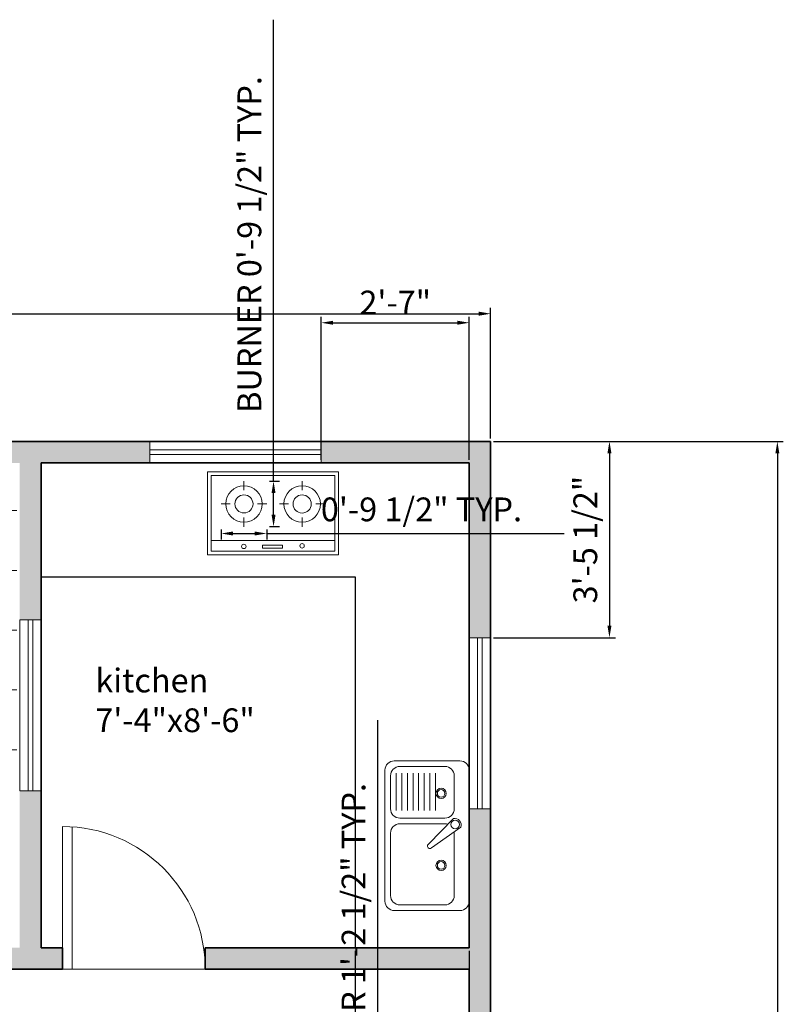
# Model space of a CAD drawing. Units: inches. Extents: x 2576 to 2974, y 2059 to 2656.
# Tile 4 of 4: x 2814 to 2974, y 2448 to 2656. Entities that reach past the tile are written whole.
import ezdxf

# ---------------------------------------------------------------- set-up
doc = ezdxf.new("R2010")
doc.units = ezdxf.units.IN
for name, color, linetype, lineweight in [('A-ANNO-DIMS', 101, 'Continuous', 18), ('A-AREA-IDEN', 101, 'Continuous', 18), ('A-EQPM', 195, 'Continuous', 18), ('A-FLOR-CASE', 143, 'Continuous', 25), ('A-FLOR-FIXT', 195, 'Continuous', 18), ('A-FLOR-PATT', 195, 'Continuous', 13), ('A-WALL-PATT', 233, 'Continuous', 13), ('doors', 235, 'Continuous', 18), ('wall', 143, 'Continuous', 35), ('windows', 85, 'Continuous', 18)]:
    doc.layers.add(name, color=color, linetype=linetype, lineweight=lineweight)
doc.styles.get("Standard").update_dxf_attribs({"font": 'txt', "height": 5})
doc.dimstyles.new('ISO-25', dxfattribs={"dimtxt": 5, "dimasz": 2.5, "dimexe": 1.25, "dimexo": 0.625, "dimtad": 1, "dimlunit": 3, "dimtxsty": 'Standard', "dimcen": 2.5, "dimadec": 0, "dimazin": 0, "dimtfac": 1, "dimtmove": 0, "dimatfit": 3, "dimfxl": 1, "dimarcsym": 0})

# ---------------------------------------------------------------- blocks, each defined once
blk = doc.blocks.new('*D2')
at = {"layer": 'A-ANNO-DIMS', "color": 0, "lineweight": -2, "transparency": 16777216}
for p, q in [((2612.56, 2567.5), (2612.56, 2595)), ((2615.06, 2593.75), (2910.06, 2593.75)), ((2912.56, 2567.5), (2912.56, 2595))]:
    blk.add_line(p, q, dxfattribs=at)
at = {"layer": 'A-ANNO-DIMS', "color": 0, "transparency": 16777216}
for points in [[(2615.06, 2594.17), (2615.06, 2593.33), (2612.56, 2593.75)], [(2910.06, 2594.17), (2910.06, 2593.33), (2912.56, 2593.75)]]:
    blk.add_solid(points, dxfattribs=at)
at = {"layer": 'Defpoints', "color": 0, "transparency": 16777216}
for p in [(2912.56, 2593.75), (2612.56, 2566.88), (2912.56, 2566.88)]:
    blk.add_point(p, dxfattribs=at)
at = {"layer": 'A-ANNO-DIMS', "color": 0, "transparency": 16777216, "insert": (2762.56, 2597.35), "char_height": 5, "attachment_point": 5}
blk.add_mtext("25'", dxfattribs=at)
blk = doc.blocks.new('*D3')
at = {"layer": 'A-ANNO-DIMS', "color": 0, "lineweight": -2, "transparency": 16777216}
for p, q in [((2913.18, 2566.88), (2974.08, 2566.88)), ((2972.83, 2564.38), (2972.83, 2089.38)), ((2913.18, 2086.88), (2974.08, 2086.88))]:
    blk.add_line(p, q, dxfattribs=at)
at = {"layer": 'A-ANNO-DIMS', "color": 0, "transparency": 16777216}
for points in [[(2972.41, 2564.38), (2973.24, 2564.38), (2972.83, 2566.88)], [(2972.41, 2089.38), (2973.24, 2089.38), (2972.83, 2086.88)]]:
    blk.add_solid(points, dxfattribs=at)
at = {"layer": 'Defpoints', "color": 0, "transparency": 16777216}
for p in [(2912.56, 2566.88), (2912.56, 2086.88), (2972.83, 2086.88)]:
    blk.add_point(p, dxfattribs=at)
at = {"layer": 'A-ANNO-DIMS', "color": 0, "transparency": 16777216, "insert": (2969.23, 2326.88), "char_height": 5, "attachment_point": 5, "rotation": 90}
blk.add_mtext("40'", dxfattribs=at)
blk = doc.blocks.new('DOOR-SWING-30IN')
for p, q in [((0, 30), (30, 30)), ((30, 30), (30, 0)), ((0.07, 28), (30, 28))]:
    blk.add_line(p, q)
blk.add_arc((30, 30), 30, 180, 270)
blk = doc.blocks.new('WINDOW-36IN')
for p, q in [((0, 36), (0, 0)), ((4.5, 36), (0, 36)), ((1.75, 36), (1.75, 0)), ((2.75, 36), (2.75, 0)), ((4.5, 0), (4.5, 36)), ((0, 0), (4.5, 0))]:
    blk.add_line(p, q)
blk = doc.blocks.new('COOKTOP-BURNER')
for p, q in [((4.79, 9.57), (4.79, 7.66)), ((0, 4.79), (1.91, 4.79)), ((7.66, 4.79), (9.57, 4.79)), ((4.79, 1.91), (4.79, 0))]:
    blk.add_line(p, q)
for radius in [3.83, 1.91]:
    blk.add_circle((4.79, 4.79), radius)
blk = doc.blocks.new('*D15')
at = {"layer": 'A-ANNO-DIMS', "color": 0, "lineweight": -2, "transparency": 16777216}
for p, q in [((2888.82, 2390.91), (2888.82, 2508.23)), ((2887.27, 2390.91), (2890.07, 2390.91)), ((2888.82, 2378.9), (2888.82, 2388.41)), ((2887.27, 2376.4), (2890.07, 2376.4))]:
    blk.add_line(p, q, dxfattribs=at)
at = {"layer": 'A-ANNO-DIMS', "color": 0, "transparency": 16777216}
for points in [[(2888.4, 2388.41), (2889.23, 2388.41), (2888.82, 2390.91)], [(2888.4, 2378.9), (2889.23, 2378.9), (2888.82, 2376.4)]]:
    blk.add_solid(points, dxfattribs=at)
at = {"layer": 'Defpoints', "color": 0, "transparency": 16777216}
for p in [(2886.64, 2390.91), (2888.82, 2390.91), (2886.64, 2376.4)]:
    blk.add_point(p, dxfattribs=at)
at = {"layer": 'A-ANNO-DIMS', "color": 0, "transparency": 16777216, "insert": (2884.38, 2450.82), "char_height": 5, "attachment_point": 5, "rotation": 90}
blk.add_mtext('DINING CHAIR 1\'-2 1/2" TYP.', dxfattribs=at)
blk = doc.blocks.new('*D17')
at = {"layer": 'A-ANNO-DIMS', "color": 0, "lineweight": -2, "transparency": 16777216}
for p, q in [((2866.92, 2558.52), (2866.92, 2655.6)), ((2866.1, 2558.52), (2868.17, 2558.52)), ((2866.92, 2551.45), (2866.92, 2556.02)), ((2866.1, 2548.95), (2868.17, 2548.95))]:
    blk.add_line(p, q, dxfattribs=at)
at = {"layer": 'A-ANNO-DIMS', "color": 0, "transparency": 16777216}
for points in [[(2866.5, 2556.02), (2867.33, 2556.02), (2866.92, 2558.52)], [(2866.5, 2551.45), (2867.33, 2551.45), (2866.92, 2548.95)]]:
    blk.add_solid(points, dxfattribs=at)
at = {"layer": 'Defpoints', "color": 0, "transparency": 16777216}
for p in [(2865.48, 2558.52), (2866.92, 2558.52), (2865.48, 2548.95)]:
    blk.add_point(p, dxfattribs=at)
at = {"layer": 'A-ANNO-DIMS', "color": 0, "transparency": 16777216, "insert": (2862.48, 2608.31), "char_height": 5, "attachment_point": 5, "rotation": 90}
blk.add_mtext('BURNER 0\'-9 1/2" TYP.', dxfattribs=at)
blk = doc.blocks.new('*D18')
at = {"layer": 'A-ANNO-DIMS', "color": 0, "lineweight": -2, "transparency": 16777216}
for p, q in [((2855.91, 2548.32), (2855.91, 2546.26)), ((2865.48, 2548.32), (2865.48, 2546.26)), ((2858.41, 2547.51), (2862.98, 2547.51)), ((2865.48, 2547.51), (2928.04, 2547.51))]:
    blk.add_line(p, q, dxfattribs=at)
at = {"layer": 'A-ANNO-DIMS', "color": 0, "transparency": 16777216}
for points in [[(2858.41, 2547.93), (2858.41, 2547.09), (2855.91, 2547.51)], [(2862.98, 2547.93), (2862.98, 2547.09), (2865.48, 2547.51)]]:
    blk.add_solid(points, dxfattribs=at)
at = {"layer": 'Defpoints', "color": 0, "transparency": 16777216}
for p in [(2855.91, 2548.95), (2865.48, 2548.95), (2865.48, 2547.51)]:
    blk.add_point(p, dxfattribs=at)
at = {"layer": 'A-ANNO-DIMS', "color": 0, "transparency": 16777216, "insert": (2898.01, 2551.94), "char_height": 5, "attachment_point": 5}
blk.add_mtext('0\'-9 1/2" TYP.', dxfattribs=at)
blk = doc.blocks.new('*D26')
at = {"layer": 'A-ANNO-DIMS', "color": 0, "lineweight": -2, "transparency": 16777216}
for p, q in [((2876.94, 2563), (2876.94, 2593.1)), ((2879.44, 2591.85), (2905.56, 2591.85)), ((2908.06, 2563), (2908.06, 2593.1))]:
    blk.add_line(p, q, dxfattribs=at)
at = {"layer": 'A-ANNO-DIMS', "color": 0, "transparency": 16777216}
for points in [[(2879.44, 2592.27), (2879.44, 2591.43), (2876.94, 2591.85)], [(2905.56, 2592.27), (2905.56, 2591.43), (2908.06, 2591.85)]]:
    blk.add_solid(points, dxfattribs=at)
at = {"layer": 'Defpoints', "color": 0, "transparency": 16777216}
for p in [(2908.06, 2591.85), (2876.94, 2562.38), (2908.06, 2562.38)]:
    blk.add_point(p, dxfattribs=at)
at = {"layer": 'A-ANNO-DIMS', "color": 0, "transparency": 16777216, "insert": (2892.5, 2595.45), "char_height": 5, "attachment_point": 5}
blk.add_mtext('2\'-7"', dxfattribs=at)
blk = doc.blocks.new('*D28')
at = {"layer": 'A-ANNO-DIMS', "color": 0, "lineweight": -2, "transparency": 16777216}
for p, q in [((2913.18, 2566.88), (2938.78, 2566.88)), ((2937.53, 2564.38), (2937.53, 2528.09)), ((2913.18, 2525.59), (2938.78, 2525.59))]:
    blk.add_line(p, q, dxfattribs=at)
at = {"layer": 'A-ANNO-DIMS', "color": 0, "transparency": 16777216}
for points in [[(2937.11, 2564.38), (2937.95, 2564.38), (2937.53, 2566.88)], [(2937.11, 2528.09), (2937.95, 2528.09), (2937.53, 2525.59)]]:
    blk.add_solid(points, dxfattribs=at)
at = {"layer": 'Defpoints', "color": 0, "transparency": 16777216}
for p in [(2912.56, 2566.88), (2912.56, 2525.59), (2937.53, 2525.59)]:
    blk.add_point(p, dxfattribs=at)
at = {"layer": 'A-ANNO-DIMS', "color": 0, "transparency": 16777216, "insert": (2933.1, 2546.23), "char_height": 5, "attachment_point": 5, "rotation": 90}
blk.add_mtext('3\'-5 1/2"', dxfattribs=at)
blk = doc.blocks.new('*D38')
at = {"layer": 'A-ANNO-DIMS', "color": 0, "lineweight": -2, "transparency": 16777216}
for p, q in [((2884.06, 2459.75), (2884.06, 2060.65)), ((2908.06, 2459.75), (2908.06, 2060.65)), ((2886.56, 2061.9), (2905.56, 2061.9))]:
    blk.add_line(p, q, dxfattribs=at)
at = {"layer": 'A-ANNO-DIMS', "color": 0, "transparency": 16777216}
for points in [[(2886.56, 2062.32), (2886.56, 2061.48), (2884.06, 2061.9)], [(2905.56, 2062.32), (2905.56, 2061.48), (2908.06, 2061.9)]]:
    blk.add_solid(points, dxfattribs=at)
at = {"layer": 'Defpoints', "color": 0, "transparency": 16777216}
for p in [(2884.06, 2460.38), (2908.06, 2460.38), (2908.06, 2061.9)]:
    blk.add_point(p, dxfattribs=at)
at = {"layer": 'A-ANNO-DIMS', "color": 0, "transparency": 16777216, "insert": (2896.06, 2065.5), "char_height": 5, "attachment_point": 5}
blk.add_mtext('2\'-0"', dxfattribs=at)

msp = doc.modelspace()

# ---------------------------------------------------------------- hatches: boundary and pattern name
at = {"layer": 'A-FLOR-PATT'}
h = msp.add_hatch(dxfattribs=at)
h.set_pattern_fill('ANGLE', color=256, scale=1.8)
h.set_pattern_definition([(0, (0, 0), (0, 12.573), [9.144, -3.429]), (90, (0, 0), (-12.573, 8e-16), [9.144, -3.429])])
h.paths.add_polyline_path([(2813.556, 2562.376), (2741.556, 2562.376), (2741.556, 2493.376), (2813.556, 2493.376), (2813.556, 2529.376)])
h.paths.add_polyline_path([(2750.035, 2495.142), (2809.21, 2495.142), (2809.21, 2502.647), (2750.035, 2502.647)], flags=24)
h.paths.add_polyline_path([(2741.924, 2553.087), (2815.278, 2553.087), (2815.278, 2560.74), (2741.924, 2560.74)], flags=9)
at = {"layer": 'A-WALL-PATT'}
h = msp.add_hatch(color=256, dxfattribs=at)
h.dxf.hatch_style = 1
h.paths.add_polyline_path([(2726.595, 2349.876), (2706.556, 2349.876), (2706.556, 2381.376), (2702.056, 2381.376), (2702.056, 2349.876), (2617.056, 2349.876), (2617.056, 2370.876), (2612.556, 2370.876), (2612.556, 2287.457), (2617.056, 2287.457), (2617.056, 2345.376), (2726.595, 2345.376)])
h.paths.add_polyline_path([(2823.556, 2345.376), (2828.056, 2345.376), (2828.056, 2349.876), (2808.018, 2349.876), (2808.018, 2345.376), (2819.056, 2345.376), (2819.056, 2206.376), (2748.056, 2206.376), (2748.056, 2201.876), (2819.056, 2201.876), (2819.056, 2159.528), (2823.556, 2159.528)])
h.paths.add_polyline_path([(2634.556, 2206.376), (2617.056, 2206.376), (2617.056, 2239.457), (2612.556, 2239.457), (2612.556, 2086.876), (2696.755, 2086.876), (2696.755, 2091.376), (2617.056, 2091.376), (2617.056, 2201.876), (2634.556, 2201.876)])
h.paths.add_polyline_path([(2688.056, 2206.376), (2670.556, 2206.376), (2670.556, 2201.876), (2688.056, 2201.876)], flags=17)
h.paths.add_polyline_path([(2832.708, 2091.376), (2732.755, 2091.376), (2732.755, 2086.876), (2832.708, 2086.876)])
h.paths.add_polyline_path([(2823.556, 2159.528), (2819.056, 2159.528), (2819.056, 2128.522), (2823.556, 2124.554)])
h.paths.add_polyline_path([(2840.936, 2566.876), (2689.889, 2566.876), (2689.889, 2562.376), (2730.206, 2562.376), (2737.056, 2562.376), (2737.056, 2529.376), (2741.556, 2529.376), (2741.556, 2562.376), (2813.556, 2562.376), (2813.556, 2529.376), (2818.056, 2529.376), (2818.056, 2562.376), (2840.936, 2562.376)])
h.paths.add_polyline_path([(2653.889, 2566.876), (2612.556, 2566.876), (2612.556, 2509.376), (2617.056, 2509.376), (2617.056, 2562.376), (2653.889, 2562.376)])
h.paths.add_polyline_path([(2822.556, 2460.376), (2818.056, 2460.376), (2818.056, 2493.376), (2813.556, 2493.376), (2813.556, 2460.376), (2809.817, 2460.376), (2809.817, 2455.876), (2822.556, 2455.876)])
h.paths.add_polyline_path([(2912.556, 2489.593), (2908.056, 2489.593), (2908.056, 2470.164), (2908.056, 2460.376), (2852.556, 2460.376), (2852.556, 2455.876), (2908.056, 2455.876), (2908.056, 2349.876), (2858.056, 2349.876), (2858.056, 2345.376), (2908.056, 2345.376), (2908.056, 2285.493), (2912.556, 2285.493)])
h.paths.add_polyline_path([(2749.817, 2460.376), (2741.556, 2460.376), (2741.556, 2493.376), (2737.056, 2493.376), (2737.056, 2450.376), (2741.556, 2450.376), (2741.556, 2455.876), (2749.817, 2455.876)])
h.paths.add_polyline_path([(2741.556, 2420.376), (2711.556, 2420.376), (2617.056, 2420.376), (2617.056, 2473.376), (2612.556, 2473.376), (2612.556, 2394.876), (2617.056, 2394.876), (2617.056, 2415.876), (2702.056, 2415.876), (2702.056, 2411.376), (2706.556, 2411.376), (2706.556, 2415.876), (2741.556, 2415.876)])
h.paths.add_polyline_path([(2912.556, 2566.876), (2876.936, 2566.876), (2876.936, 2562.376), (2908.056, 2562.376), (2908.056, 2525.593), (2912.556, 2525.593)])
h.paths.add_polyline_path([(2741.924, 2553.087), (2815.278, 2553.087), (2815.278, 2560.74), (2741.924, 2560.74)], flags=25)

# ---------------------------------------------------------------- linework, layer by layer
at = {"layer": 'A-EQPM'}
for p, q in [((2853.037, 2560.51), (2853.037, 2543.01)), ((2853.037, 2560.51), (2880.593, 2560.51)), ((2880.593, 2560.51), (2880.593, 2543.01)), ((2853.803, 2559.744), (2853.803, 2543.776)), ((2853.803, 2559.744), (2879.828, 2559.744)), ((2879.828, 2559.744), (2879.828, 2543.776)), ((2853.803, 2546.073), (2879.828, 2546.073)), ((2853.803, 2543.776), (2879.828, 2543.776)), ((2864.589, 2545.054), (2868.81, 2545.054)), ((2864.589, 2544.447), (2864.589, 2545.054)), ((2868.81, 2544.447), (2864.589, 2544.447)), ((2868.81, 2545.054), (2868.81, 2544.447)), ((2853.037, 2543.01), (2880.593, 2543.01))]:
    msp.add_line(p, q, dxfattribs=at)
for centre in [(2860.672, 2544.784), (2872.928, 2544.919)]:
    msp.add_circle(centre, 0.459, dxfattribs=at)
at = {"layer": 'A-FLOR-CASE'}
for p, q in [((2818.056, 2538.376), (2884.056, 2538.376)), ((2884.056, 2538.376), (2884.056, 2460.376))]:
    msp.add_line(p, q, dxfattribs=at)
at = {"layer": 'A-FLOR-FIXT'}
for p, q in [((2906.088, 2499.691), (2892.308, 2499.691)), ((2902.938, 2498.51), (2893.489, 2498.51)), ((2890.34, 2497.723), (2890.34, 2470.164)), ((2891.521, 2496.542), (2891.521, 2489.601)), ((2892.695, 2489.215), (2892.695, 2497.104)), ((2893.876, 2489.215), (2893.876, 2497.104)), ((2895.058, 2489.215), (2895.058, 2497.104)), ((2896.239, 2489.215), (2896.239, 2497.104)), ((2897.42, 2489.215), (2897.42, 2497.104)), ((2898.601, 2489.215), (2898.601, 2497.104)), ((2899.782, 2489.215), (2899.782, 2497.104)), ((2900.963, 2489.215), (2900.963, 2497.104)), ((2904.907, 2496.542), (2904.907, 2489.601)), ((2908.056, 2470.164), (2908.056, 2497.723)), ((2902.938, 2487.632), (2893.489, 2487.632)), ((2902.938, 2486.451), (2893.489, 2486.451)), ((2904.755, 2487.545), (2899.466, 2482.167)), ((2906.291, 2485.749), (2900.156, 2481.361)), ((2891.521, 2484.483), (2891.521, 2471.345)), ((2904.907, 2471.345), (2904.907, 2484.483)), ((2893.489, 2469.376), (2902.938, 2469.376)), ((2892.308, 2468.195), (2906.088, 2468.195))]:
    msp.add_line(p, q, dxfattribs=at)
for centre, radius in [((2902.145, 2492.844), 1.081), ((2902.145, 2492.844), 0.788), ((2905.104, 2486.289), 0.892), ((2902.145, 2477.698), 1.081), ((2902.145, 2477.698), 0.788)]:
    msp.add_circle(centre, radius, dxfattribs=at)
for centre, radius, start, end in [((2892.308, 2497.723), 1.968, 90, 180), ((2893.489, 2496.542), 1.968, 90, 180), ((2902.938, 2496.542), 1.968, 0, 90), ((2906.088, 2497.723), 1.968, 0, 90), ((2893.489, 2489.601), 1.968, 180, 270), ((2902.938, 2489.601), 1.968, 270, 0), ((2893.489, 2484.483), 1.968, 90, 180), ((2902.938, 2484.483), 1.968, 71.10956, 90), ((2905.005, 2486.204), 1.364, 340.52706, 100.52706), ((2902.938, 2484.483), 1.968, 0, 7.6978), ((2899.805, 2481.759), 0.531, 129.73777, 311.31634), ((2893.489, 2471.345), 1.968, 180, 270), ((2902.938, 2471.345), 1.968, 270, 0), ((2892.308, 2470.164), 1.968, 180, 270), ((2906.088, 2470.164), 1.968, 270, 0)]:
    msp.add_arc(centre, radius, start, end, dxfattribs=at)
at = {"layer": 'wall'}
for p, q in [((2612.556, 2566.876), (2912.556, 2566.876)), ((2912.556, 2566.876), (2912.556, 2086.876)), ((2818.056, 2460.376), (2818.056, 2562.376)), ((2818.056, 2562.376), (2908.056, 2562.376)), ((2908.056, 2562.376), (2908.056, 2460.376)), ((2818.056, 2460.376), (2822.556, 2460.376)), ((2822.556, 2460.376), (2822.556, 2455.876)), ((2852.556, 2460.376), (2852.556, 2455.876)), ((2852.556, 2460.376), (2908.056, 2460.376)), ((2809.817, 2455.876), (2822.556, 2455.876)), ((2852.556, 2455.876), (2908.056, 2455.876)), ((2908.056, 2455.876), (2908.056, 2349.876))]:
    msp.add_line(p, q, dxfattribs=at)

# ---------------------------------------------------------------- block references
at = {"layer": 'A-EQPM'}
msp.add_blockref('COOKTOP-BURNER', (2855.908, 2548.946), dxfattribs=at)
at = {"layer": 'A-EQPM', "rotation": 180}
msp.add_blockref('COOKTOP-BURNER', (2877.722, 2558.516), dxfattribs=at)
at = {"layer": 'doors', "extrusion": (0, 0, -1), "zscale": -1, "rotation": 270.0000000000124}
msp.add_blockref('DOOR-SWING-30IN', (-2852.556, 2485.876), dxfattribs=at)
at = {"layer": 'windows', "rotation": 89.99999999999874}
msp.add_blockref('WINDOW-36IN', (2876.936, 2562.376), dxfattribs=at)
at = {"layer": 'windows'}
for p in [(2813.556, 2493.376), (2908.056, 2489.593)]:
    msp.add_blockref('WINDOW-36IN', p, dxfattribs=at)

# ---------------------------------------------------------------- texts
at = {"layer": 'A-AREA-IDEN'}
for s, p in [('kitchen', (2829.443, 2514.089)), ('7\'-4"x8\'-6"', (2829.443, 2505.72))]:
    msp.add_text(s, height=5, dxfattribs=at).set_placement(p)

# ---------------------------------------------------------------- dimensions: what is measured, and where the dimension line sits
at = {"layer": 'A-ANNO-DIMS'}
for base, p1, p2, text, picture, middle in [((2866.915, 2558.516), (2865.479, 2548.946), (2865.479, 2558.516), 'BURNER <> TYP.', '*D17', (2862.48, 2608.308)), ((2888.816, 2390.906), (2886.641, 2376.402), (2886.641, 2390.906), 'DINING CHAIR <> TYP.', '*D15', (2884.382, 2450.816))]:
    dim = msp.add_linear_dim(base=base, p1=p1, p2=p2, angle=90, text=text, dimstyle='ISO-25', override={"dimdec": 1, "dimlfac": 1, "dimrnd": 0, "dimzin": 1, "dimdsep": 46, "dimlunit": 4, "dimfrac": 2}, dxfattribs=at)
    dim.commit()
    dim.dimension.update_dxf_attribs({"geometry": picture, "text_midpoint": middle})
for base, p1, p2, override, picture, middle in [((2912.556, 2593.75), (2612.556, 2566.876), (2912.556, 2566.876), {"dimclrd": 0, "dimclre": 0, "dimclrt": 0}, '*D2', (2762.556, 2597.351)), ((2908.056, 2591.851), (2876.936, 2562.376), (2908.056, 2562.376), {"dimdec": 1, "dimlfac": 1, "dimrnd": 0, "dimzin": 1, "dimdsep": 46, "dimlunit": 4, "dimfrac": 2}, '*D26', (2892.496, 2595.452)), ((2908.056, 2061.901), (2884.056, 2460.376), (2908.056, 2460.376), {"dimdec": 1, "dimlfac": 1, "dimrnd": 0, "dimzin": 1, "dimdsep": 46, "dimlunit": 4, "dimfrac": 2}, '*D38', (2896.056, 2065.502))]:
    dim = msp.add_linear_dim(base=base, p1=p1, p2=p2, dimstyle='ISO-25', override=override, dxfattribs=at)
    dim.commit()
    dim.dimension.update_dxf_attribs({"geometry": picture, "text_midpoint": middle})
for base, p2, override, picture, middle in [((2972.827, 2086.876), (2912.556, 2086.876), {"dimclrd": 0, "dimclre": 0, "dimclrt": 0}, '*D3', (2969.226, 2326.876)), ((2937.531, 2525.593), (2912.556, 2525.593), {"dimdec": 1, "dimlfac": 1, "dimrnd": 0, "dimzin": 1, "dimdsep": 46, "dimlunit": 4, "dimfrac": 2}, '*D28', (2933.097, 2546.234))]:
    dim = msp.add_linear_dim(base=base, p1=(2912.556, 2566.876), p2=p2, angle=90, dimstyle='ISO-25', override=override, dxfattribs=at)
    dim.commit()
    dim.dimension.update_dxf_attribs({"geometry": picture, "text_midpoint": middle})
dim = msp.add_linear_dim(base=(2865.479, 2547.51), p1=(2855.908, 2548.946), p2=(2865.479, 2548.946), text='<> TYP.', dimstyle='ISO-25', override={"dimdec": 1, "dimlfac": 1, "dimrnd": 0, "dimzin": 1, "dimdsep": 46, "dimlunit": 4, "dimfrac": 2}, dxfattribs=at)
dim.commit()
dim.dimension.update_dxf_attribs({"geometry": '*D18', "text_midpoint": (2898.009, 2551.944)})

doc.saveas('drawing.dxf')
